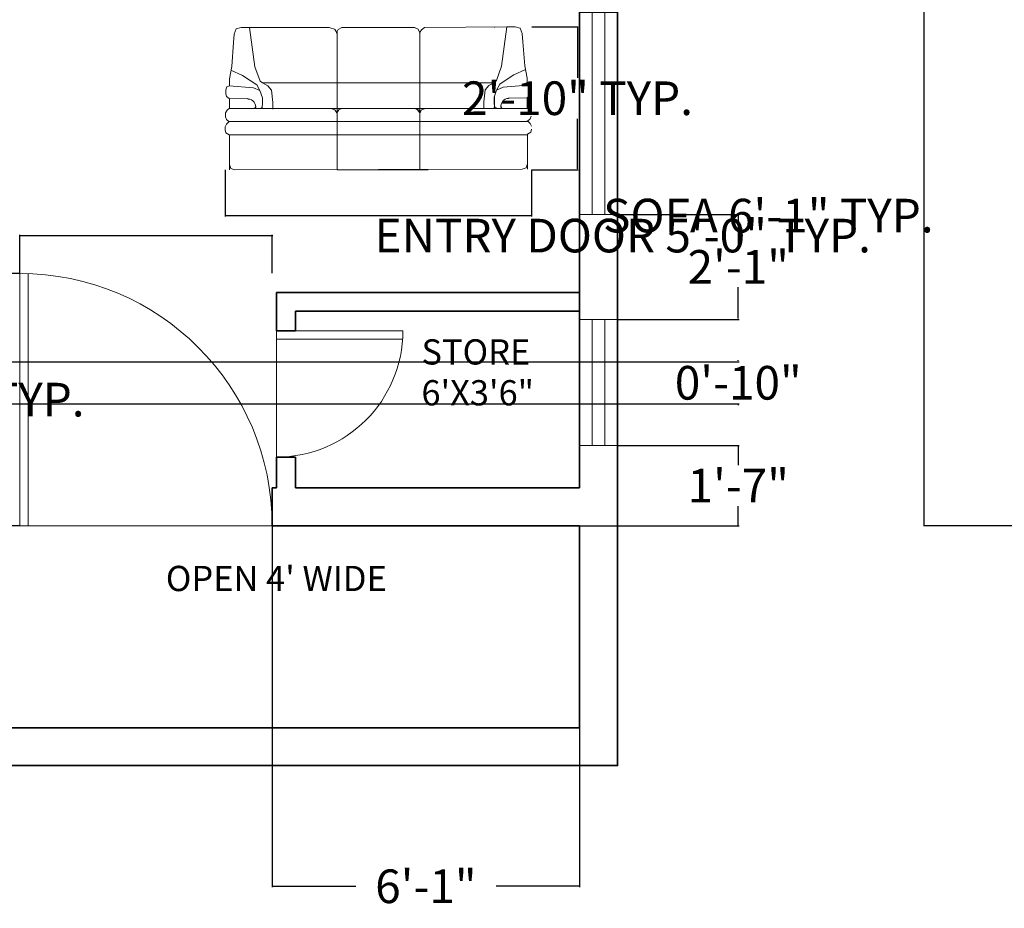
# Model space of a CAD drawing. Units: inches. Extents: x 125 to 976, y 231 to 853.
# Tile 4 of 16: x 324 to 557, y 238 to 449. Entities that reach past the tile are written whole.
import ezdxf

# ---------------------------------------------------------------- set-up
doc = ezdxf.new("R2010")
doc.units = ezdxf.units.IN
doc.header["$MEASUREMENT"] = 0
for name, color, linetype, lineweight in [('A-ANNO-DIMS', 2, 'Continuous', 18), ('A-AREA-IDEN', 7, 'Continuous', 18), ('A-DOOR', 3, 'Continuous', 18), ('A-GLAZ', 4, 'Continuous', 18), ('A-WALL', 7, 'Continuous', 35), ('Furniture', 8, 'Continuous', 15)]:
    doc.layers.add(name, color=color, linetype=linetype, lineweight=lineweight)
doc.styles.get("Standard").update_dxf_attribs({"font": 'italic8.shx'})
doc.dimstyles.get("Standard").update_dxf_attribs({"dimtxt": 8, "dimasz": 0.18, "dimexe": 0.18, "dimexo": 0.0625, "dimgap": 0.09, "dimtad": 0, "dimtih": 1, "dimtoh": 1, "dimdec": 4, "dimzin": 0, "dimdsep": 46, "dimlunit": 3, "dimtxsty": 'Standard', "dimcen": 0.09, "dimclrt": 4, "dimadec": 0, "dimazin": 0, "dimtfac": 1, "dimtdec": 4, "dimtofl": 0, "dimtmove": 0, "dimatfit": 3, "dimfxl": 1, "dimtolj": 1, "dimtzin": 0, "dimarcsym": 0})

# ---------------------------------------------------------------- blocks, each defined once
blk = doc.blocks.new('SOFA-3SEAT')
for p, q in [((2.15, 32.26, -13.5), (2.61, 33.47, -13.5)), ((2.61, 33.47, -13.5), (3.76, 33.83, -13.5)), ((3.76, 33.83, -13.5), (5.77, 33.83, -13.5)), ((5.77, 33.83, -13.5), (24.71, 33.77, -13.5)), ((5.77, 33.83, -13.5), (7.07, 24.49, -13.5)), ((24.71, 33.77, -13.5), (26.18, 33.35, -13.5)), ((26.04, 33.37, -13.5), (26.5, 32.59, -13.5)), ((26.43, 32.53, -13.5), (26.87, 33.35, -13.5)), ((26.58, 32.81, -13.5), (26.58, 0, -13.5)), ((26.87, 33.35, -13.5), (27.73, 33.77, -13.5)), ((27.73, 33.77, -13.5), (44.96, 33.81, -13.5)), ((45.83, 33.4, -13.5), (44.96, 33.81, -13.5)), ((46.26, 32.57, -13.5), (45.83, 33.4, -13.5)), ((46.26, 32.63, -13.5), (46.69, 33.25, -13.5)), ((46.69, 33.25, -13.5), (47.38, 33.77, -13.5)), ((47.38, 33.77, -13.5), (66.92, 33.97, -13.5)), ((63.98, 33.86, -13.5), (63.98, 33.83, -13.5)), ((66.92, 33.97, -13.5), (65.66, 24.62, -13.5)), ((68.93, 33.98, -13.5), (66.92, 33.97, -13.5)), ((70.09, 33.62, -13.5), (68.93, 33.98, -13.5)), ((70.54, 32.42, -13.5), (70.09, 33.62, -13.5)), ((2, 30.21, -13.5), (2.15, 32.26, -13.5)), ((26.46, 32.58, -13.5), (26.52, 32.42, -13.5)), ((46.23, 32.63, -13.5), (46.18, 32.47, -13.5)), ((46.27, 0, -13.5), (46.27, 32.64, -13.5)), ((70.7, 30.37, -13.5), (70.54, 32.42, -13.5)), ((1.55, 24.55, -13.5), (2, 30.21, -13.5)), ((71.18, 24.71, -13.5), (70.7, 30.37, -13.5)), ((0.99, 21.59, -13.5), (1.55, 24.55, -13.5)), ((1.35, 23.64, -13.5), (4.11, 22.38, -13.5)), ((7.07, 24.49, -13.5), (8.28, 21.05, -13.5)), ((65.66, 24.62, -13.5), (64.47, 21.18, -13.5)), ((71.39, 23.81, -13.5), (68.63, 22.53, -13.5)), ((71.76, 21.75, -13.5), (71.18, 24.71, -13.5)), ((0.99, 21.59, -13.5), (0.99, 19.94, -13.5)), ((4.11, 22.38, -13.5), (5.97, 21.23, -13.5)), ((5.97, 21.23, -13.5), (7.53, 20.21, -13.5)), ((64.47, 21.18, -13.5), (63.92, 20.76, -13.5)), ((66.78, 21.37, -13.5), (65.23, 20.34, -13.5)), ((68.63, 22.53, -13.5), (66.78, 21.37, -13.5)), ((71.76, 21.75, -13.5), (71.76, 20.1, -13.5)), ((0.14, 18.15, -13.5), (0.18, 18.99, -13.5)), ((0.18, 18.99, -13.5), (0.38, 19.7, -13.5)), ((0.38, 19.7, -13.5), (0.98, 19.91, -13.5)), ((0.65, 19.79, -13.5), (0.65, 19.8, -13.5)), ((0.96, 19.94, -13.5), (6.7, 19.5, -13.5)), ((6.7, 19.5, -13.5), (8.26, 18.79, -13.5)), ((7.53, 20.21, -13.5), (8.33, 18.64, -13.5)), ((8.26, 18.79, -13.5), (8.83, 17.11, -13.5)), ((8.28, 21.05, -13.5), (8.83, 20.63, -13.5)), ((8.83, 20.63, -13.5), (63.95, 20.63, -13.5)), ((8.83, 20.63, -13.5), (10.14, 19.91, -13.5)), ((8.86, 20.63, -13.5), (8.86, 20.61, -13.5)), ((10.14, 19.91, -13.5), (10.98, 18.9, -13.5)), ((10.98, 18.9, -13.5), (11.34, 16.01, -13.5)), ((61.78, 19.02, -13.5), (61.43, 16.13, -13.5)), ((62.62, 20.03, -13.5), (61.78, 19.02, -13.5)), ((63.92, 20.76, -13.5), (62.62, 20.03, -13.5)), ((63.89, 20.76, -13.5), (63.89, 20.74, -13.5)), ((64.5, 18.92, -13.5), (63.94, 17.24, -13.5)), ((65.23, 20.34, -13.5), (64.43, 18.77, -13.5)), ((66.05, 19.64, -13.5), (64.5, 18.92, -13.5)), ((71.8, 20.1, -13.5), (66.05, 19.64, -13.5)), ((72.37, 19.87, -13.5), (71.78, 20.07, -13.5)), ((72.11, 19.95, -13.5), (72.11, 19.96, -13.5)), ((72.58, 19.16, -13.5), (72.37, 19.87, -13.5)), ((72.62, 18.32, -13.5), (72.58, 19.16, -13.5)), ((0.35, 17.44, -13.5), (0.14, 18.15, -13.5)), ((0.98, 16.94, -13.5), (0.35, 17.44, -13.5)), ((0.98, 16.95, -13.5), (5.28, 16.85, -13.5)), ((0.99, 16.95, -13.5), (0.99, 14.57, -13.5)), ((0.99, 14.57, -13.5), (0.99, 16.93, -13.5)), ((5.51, 16.75, -13.5), (5.27, 16.91, -13.5)), ((8.83, 17.11, -13.5), (8.86, 15.72, -13.5)), ((63.94, 17.24, -13.5), (63.91, 15.85, -13.5)), ((63.98, 17.37, -13.5), (63.98, 14.57, -13.5)), ((67.26, 16.9, -13.5), (67.49, 17.06, -13.5)), ((71.79, 17.11, -13.5), (67.48, 17, -13.5)), ((71.78, 17.11, -13.5), (71.79, 14.73, -13.5)), ((71.79, 14.73, -13.5), (71.78, 17.09, -13.5)), ((71.79, 17.1, -13.5), (72.41, 17.61, -13.5)), ((71.86, 17.15, -13.5), (71.86, 14.57, -13.5)), ((72.41, 17.61, -13.5), (72.62, 18.32, -13.5)), ((0.04, 13.5, -13.5), (0.49, 14.17, -13.5)), ((0.49, 14.17, -13.5), (1.01, 14.59, -13.5)), ((0.99, 14.57, -13.5), (71.86, 14.57, -13.5)), ((0.99, 14.57, -13.5), (0.99, 14.57, -13.5)), ((7.07, 14.84, -13.5), (7.3, 14.56, -13.5)), ((8.66, 14.72, -13.5), (8.26, 14.56, -13.5)), ((8.83, 14.88, -13.5), (8.66, 14.72, -13.5)), ((8.86, 15.75, -13.5), (8.81, 14.86, -13.5)), ((8.89, 14.57, -13.5), (8.89, 14.52, -13.5)), ((11.34, 16.01, -13.5), (11.34, 14.42, -13.5)), ((25.14, 14.53, -13.5), (26.09, 14.22, -13.5)), ((26.09, 14.22, -13.5), (26.52, 13.5, -13.5)), ((26.52, 13.5, -13.5), (27.04, 14.22, -13.5)), ((27.04, 14.22, -13.5), (27.73, 14.53, -13.5)), ((45.74, 14.26, -13.5), (45.05, 14.57, -13.5)), ((45.14, 14.53, -13.5), (46.17, 14.12, -13.5)), ((46.26, 13.54, -13.5), (45.74, 14.26, -13.5)), ((46.17, 14.12, -13.5), (46.26, 13.39, -13.5)), ((46.69, 14.27, -13.5), (46.26, 13.54, -13.5)), ((46.26, 13.39, -13.5), (46.6, 14.12, -13.5)), ((46.6, 14.12, -13.5), (47.29, 14.53, -13.5)), ((47.64, 14.58, -13.5), (46.69, 14.27, -13.5)), ((61.43, 16.13, -13.5), (61.44, 14.54, -13.5)), ((63.88, 14.69, -13.5), (63.88, 14.65, -13.5)), ((63.91, 15.87, -13.5), (63.97, 14.99, -13.5)), ((63.95, 15.01, -13.5), (64.12, 14.85, -13.5)), ((64.12, 14.85, -13.5), (64.51, 14.69, -13.5)), ((65.71, 14.98, -13.5), (65.48, 14.7, -13.5)), ((72.29, 14.34, -13.5), (71.76, 14.75, -13.5)), ((71.79, 14.73, -13.5), (71.79, 14.74, -13.5)), ((72.75, 13.67, -13.5), (72.29, 14.34, -13.5)), ((0.04, 12.58, -13.5), (0.04, 13.5, -13.5)), ((0.31, 11.91, -13.5), (0.04, 12.58, -13.5)), ((0.98, 11.41, -13.5), (0.31, 11.91, -13.5)), ((71.81, 11.57, -13.5), (72.48, 12.08, -13.5)), ((72.48, 12.08, -13.5), (72.75, 12.75, -13.5)), ((0.31, 10.84, -13.5), (0, 10.18, -13.5)), ((0, 10.18, -13.5), (0, 9.47, -13.5)), ((0, 9.47, -13.5), (0.19, 8.77, -13.5)), ((0.98, 11.45, -13.5), (0.31, 10.84, -13.5)), ((71.86, 11.42, -13.5), (0.99, 11.42, -13.5)), ((71.8, 11.42, -13.5), (71.8, 11.58, -13.5)), ((71.82, 11.61, -13.5), (72.49, 11, -13.5)), ((71.86, 11.6, -13.5), (71.86, 11.42, -13.5)), ((71.86, 11.6, -13.5), (71.86, 11.42, -13.5)), ((72.49, 11, -13.5), (72.8, 10.35, -13.5)), ((72.81, 9.64, -13.5), (72.61, 8.93, -13.5)), ((0.19, 8.77, -13.5), (0.98, 8.25, -13.5)), ((0.99, 8.27, -13.5), (71.86, 8.27, -13.5)), ((0.99, 0, -13.5), (0.99, 8.27, -13.5)), ((0.99, 8.27, -13.5), (0.99, 1.21, -13.5)), ((0.99, 8.27, -13.5), (0.99, 0, -13.5)), ((71.82, 8.43, -13.5), (71.81, 8.27, -13.5)), ((71.86, 0.16, -13.5), (71.82, 8.43, -13.5)), ((71.82, 8.43, -13.5), (71.85, 1.37, -13.5)), ((71.86, 0.16, -13.5), (71.82, 8.27, -13.5)), ((72.61, 8.93, -13.5), (71.83, 8.41, -13.5)), ((71.86, 8.43, -13.5), (71.86, 8.27, -13.5)), ((0.99, 1.21, -13.5), (1.35, 0.26, -13.5)), ((1.35, 0.26, -13.5), (2.3, 0, -13.5)), ((2.3, 0, -13.5), (70.55, 0.16, -13.5)), ((71.49, 0.42, -13.5), (70.55, 0.16, -13.5)), ((71.85, 1.37, -13.5), (71.49, 0.42, -13.5)), ((26.58, 0, -13.5), (46.27, 0, -13.5)), ((28.55, 0, -13.5), (48.23, 0, -13.5))]:
    blk.add_line(p, q)
for centre, start, end in [((5.4, 14.95, -13.5), 347.9294, 88.2763), ((67.38, 15.1, -13.5), 91.9867, 192.3335)]:
    blk.add_arc(centre, 1.85, start, end)
blk = doc.blocks.new('WINDOW-48IN')
for p, q in [((0, 0), (0, 48)), ((0, 48), (9, 48)), ((3, 0), (3, 48)), ((6, 0), (6, 48)), ((9, 48), (9, 0)), ((9, 0), (0, 0))]:
    blk.add_line(p, q)
blk = doc.blocks.new('WINDOW-30IN')
for p, q in [((0, 0), (0, 9)), ((0, 9), (30, 9)), ((30, 9), (30, 0)), ((30, 6), (0, 6)), ((30, 3), (0, 3)), ((30, 0), (0, 0))]:
    blk.add_line(p, q)
blk = doc.blocks.new('DOOR-30IN')
for p, q in [((-2, 29.93), (-2, 0)), ((0, 30), (0, 0)), ((0, 0), (-30, 0))]:
    blk.add_line(p, q)
blk.add_arc((0, 0), 30, 90, 180)
blk = doc.blocks.new('DOOR-60IN')
for p, q in [((0, 0), (0, 60)), ((2, 0), (2, 59.97)), ((60, 0), (0, 0))]:
    blk.add_line(p, q)
blk.add_arc((0, 0), 60, 0, 90)
blk = doc.blocks.new('*D42')
at = {"layer": 'A-ANNO-DIMS', "color": 0, "lineweight": -2, "transparency": 16777216}
for p, q in [((372.34, 413.71), (372.34, 402.67)), ((445.15, 413.71), (445.15, 402.67)), ((372.52, 402.85), (444.97, 402.85)), ((445.15, 402.85), (445.33, 402.85))]:
    blk.add_line(p, q, dxfattribs=at)
at = {"layer": 'A-ANNO-DIMS', "color": 0, "transparency": 16777216}
for points in [[(372.52, 402.88), (372.52, 402.82), (372.34, 402.85)], [(444.97, 402.88), (444.97, 402.82), (445.15, 402.85)]]:
    blk.add_solid(points, dxfattribs=at)
at = {"layer": 'Defpoints', "color": 0, "transparency": 16777216}
for p in [(372.34, 413.77), (445.15, 413.77), (445.15, 402.85)]:
    blk.add_point(p, dxfattribs=at)
at = {"layer": 'A-ANNO-DIMS', "color": 4, "transparency": 16777216, "insert": (501.42, 402.85), "char_height": 8, "attachment_point": 5}
blk.add_mtext('\\A1;SOFA 6\'-1" TYP.', dxfattribs=at)
blk = doc.blocks.new('*D43')
at = {"layer": 'A-ANNO-DIMS', "color": 0, "lineweight": -2, "transparency": 16777216}
for p, q in [((445.21, 447.74), (456.25, 447.74)), ((456.07, 447.56), (456.07, 435.61)), ((456.07, 413.95), (456.07, 425.9)), ((445.21, 413.77), (456.25, 413.77))]:
    blk.add_line(p, q, dxfattribs=at)
at = {"layer": 'A-ANNO-DIMS', "color": 0, "transparency": 16777216}
for points in [[(456.04, 447.56), (456.1, 447.56), (456.07, 447.74)], [(456.04, 413.95), (456.1, 413.95), (456.07, 413.77)]]:
    blk.add_solid(points, dxfattribs=at)
at = {"layer": 'Defpoints', "color": 0, "transparency": 16777216}
for p in [(445.15, 447.74), (456.07, 447.74), (445.15, 413.77)]:
    blk.add_point(p, dxfattribs=at)
at = {"layer": 'A-ANNO-DIMS', "color": 4, "transparency": 16777216, "insert": (456.07, 430.76), "char_height": 8, "attachment_point": 5}
blk.add_mtext('\\A1;2\'-10" TYP.', dxfattribs=at)
blk = doc.blocks.new('*D54')
at = {"layer": 'A-ANNO-DIMS', "color": 0, "lineweight": -2, "transparency": 16777216}
for p, q in [((323.51, 389.17), (323.51, 398.28)), ((323.69, 398.1), (383.33, 398.1)), ((383.51, 389.17), (383.51, 398.28)), ((383.51, 398.1), (383.69, 398.1))]:
    blk.add_line(p, q, dxfattribs=at)
at = {"layer": 'A-ANNO-DIMS', "color": 0, "transparency": 16777216}
for points in [[(323.69, 398.13), (323.69, 398.07), (323.51, 398.1)], [(383.33, 398.13), (383.33, 398.07), (383.51, 398.1)]]:
    blk.add_solid(points, dxfattribs=at)
at = {"layer": 'Defpoints', "color": 0, "transparency": 16777216}
for p in [(383.51, 398.1), (323.51, 389.1), (383.51, 389.1)]:
    blk.add_point(p, dxfattribs=at)
at = {"layer": 'A-ANNO-DIMS', "color": 4, "transparency": 16777216, "insert": (466.83, 398.1), "char_height": 8, "attachment_point": 5}
blk.add_mtext('\\A1;ENTRY DOOR 5\'-0" TYP.', dxfattribs=at)
blk = doc.blocks.new('*D55')
at = {"layer": 'A-ANNO-DIMS', "color": 0, "lineweight": -2, "transparency": 16777216}
for p, q in [((323.45, 389.1), (314.33, 389.1)), ((314.51, 388.92), (314.51, 363.96)), ((314.51, 329.28), (314.51, 354.25)), ((323.45, 329.1), (314.33, 329.1))]:
    blk.add_line(p, q, dxfattribs=at)
at = {"layer": 'A-ANNO-DIMS', "color": 0, "transparency": 16777216}
for points in [[(314.48, 388.92), (314.54, 388.92), (314.51, 389.1)], [(314.48, 329.28), (314.54, 329.28), (314.51, 329.1)]]:
    blk.add_solid(points, dxfattribs=at)
at = {"layer": 'Defpoints', "color": 0, "transparency": 16777216}
for p in [(314.51, 389.1), (323.51, 389.1), (323.51, 329.1)]:
    blk.add_point(p, dxfattribs=at)
at = {"layer": 'A-ANNO-DIMS', "color": 4, "transparency": 16777216, "insert": (314.51, 359.1), "char_height": 8, "attachment_point": 5}
blk.add_mtext('\\A1;5\'-0" TYP.', dxfattribs=at)
blk = doc.blocks.new('*D57')
at = {"layer": 'A-ANNO-DIMS', "color": 0, "lineweight": -2, "transparency": 16777216}
for p, q in [((567.13, 812.1), (538.31, 812.1)), ((538.49, 811.92), (538.49, 575.46)), ((538.49, 329.28), (538.49, 565.75)), ((576.13, 329.1), (538.31, 329.1))]:
    blk.add_line(p, q, dxfattribs=at)
at = {"layer": 'A-ANNO-DIMS', "color": 0, "transparency": 16777216}
for points in [[(538.46, 811.92), (538.52, 811.92), (538.49, 812.1)], [(538.46, 329.28), (538.52, 329.28), (538.49, 329.1)]]:
    blk.add_solid(points, dxfattribs=at)
at = {"layer": 'Defpoints', "color": 0, "transparency": 16777216}
for p in [(538.49, 812.1), (567.19, 812.1), (576.19, 329.1)]:
    blk.add_point(p, dxfattribs=at)
at = {"layer": 'A-ANNO-DIMS', "color": 4, "transparency": 16777216, "insert": (538.49, 570.6), "char_height": 8, "attachment_point": 5}
blk.add_mtext('\\A1;40\'-3"', dxfattribs=at)
blk = doc.blocks.new('*D59')
at = {"layer": 'A-ANNO-DIMS', "color": 0, "lineweight": -2, "transparency": 16777216}
for p, q in [((222.641698, 368.104746), (494.459198, 368.104746)), ((494.279198, 368.284746), (494.279198, 368.464746)), ((222.641698, 358.104746), (494.459198, 358.104746)), ((494.279198, 357.924746), (494.279198, 357.744746))]:
    blk.add_line(p, q, dxfattribs=at)
at = {"layer": 'A-ANNO-DIMS', "color": 0, "transparency": 16777216}
for points in [[(494.249198, 368.284746), (494.309198, 368.284746), (494.279198, 368.104746)], [(494.249198, 357.924746), (494.309198, 357.924746), (494.279198, 358.104746)]]:
    blk.add_solid(points, dxfattribs=at)
at = {"layer": 'Defpoints', "color": 0, "transparency": 16777216}
for p in [(222.579198, 368.104746), (494.279198, 368.104746), (222.579198, 358.104746)]:
    blk.add_point(p, dxfattribs=at)
at = {"layer": 'A-ANNO-DIMS', "color": 4, "transparency": 16777216, "insert": (494.279198, 363.104746), "char_height": 8, "attachment_point": 5}
blk.add_mtext('\\A1;0\'-10"', dxfattribs=at)
blk = doc.blocks.new('*D60')
at = {"layer": 'A-ANNO-DIMS', "color": 0, "lineweight": -2, "transparency": 16777216}
for p, q in [((383.51, 329.04), (383.51, 243.22)), ((456.58, 329.04), (456.58, 243.22)), ((383.69, 243.4), (403.39, 243.4)), ((456.4, 243.4), (436.71, 243.4))]:
    blk.add_line(p, q, dxfattribs=at)
at = {"layer": 'A-ANNO-DIMS', "color": 0, "transparency": 16777216}
for points in [[(383.69, 243.43), (383.69, 243.37), (383.51, 243.4)], [(456.4, 243.43), (456.4, 243.37), (456.58, 243.4)]]:
    blk.add_solid(points, dxfattribs=at)
at = {"layer": 'Defpoints', "color": 0, "transparency": 16777216}
for p in [(383.51, 329.1), (456.58, 329.1), (456.58, 243.4)]:
    blk.add_point(p, dxfattribs=at)
at = {"layer": 'A-ANNO-DIMS', "color": 4, "transparency": 16777216, "insert": (420.05, 243.4), "char_height": 8, "attachment_point": 5}
blk.add_mtext('\\A1;6\'-1"', dxfattribs=at)
blk = doc.blocks.new('*D62')
at = {"layer": 'A-ANNO-DIMS', "color": 0, "lineweight": -2, "transparency": 16777216}
for p, q in [((465.64, 348.19), (494.46, 348.19)), ((494.28, 348.01), (494.28, 343.5)), ((494.28, 329.28), (494.28, 333.79)), ((456.64, 329.1), (494.46, 329.1))]:
    blk.add_line(p, q, dxfattribs=at)
at = {"layer": 'A-ANNO-DIMS', "color": 0, "transparency": 16777216}
for points in [[(494.25, 348.01), (494.31, 348.01), (494.28, 348.19)], [(494.25, 329.28), (494.31, 329.28), (494.28, 329.1)]]:
    blk.add_solid(points, dxfattribs=at)
at = {"layer": 'Defpoints', "color": 0, "transparency": 16777216}
for p in [(465.58, 348.19), (494.28, 348.19), (456.58, 329.1)]:
    blk.add_point(p, dxfattribs=at)
at = {"layer": 'A-ANNO-DIMS', "color": 4, "transparency": 16777216, "insert": (494.28, 338.65), "char_height": 8, "attachment_point": 5}
blk.add_mtext('\\A1;1\'-7"', dxfattribs=at)
blk = doc.blocks.new('*D63')
at = {"layer": 'A-ANNO-DIMS', "color": 0, "lineweight": -2, "transparency": 16777216}
for p, q in [((465.64, 403.13), (494.46, 403.13)), ((494.28, 402.95), (494.28, 395.51)), ((494.28, 378.37), (494.28, 385.8)), ((465.64, 378.19), (494.46, 378.19))]:
    blk.add_line(p, q, dxfattribs=at)
at = {"layer": 'A-ANNO-DIMS', "color": 0, "transparency": 16777216}
for points in [[(494.25, 402.95), (494.31, 402.95), (494.28, 403.13)], [(494.25, 378.37), (494.31, 378.37), (494.28, 378.19)]]:
    blk.add_solid(points, dxfattribs=at)
at = {"layer": 'Defpoints', "color": 0, "transparency": 16777216}
for p in [(465.58, 403.13), (494.28, 403.13), (465.58, 378.19)]:
    blk.add_point(p, dxfattribs=at)
at = {"layer": 'A-ANNO-DIMS', "color": 4, "transparency": 16777216, "insert": (494.28, 390.66), "char_height": 8, "attachment_point": 5}
blk.add_mtext('\\A1;2\'-1"', dxfattribs=at)

msp = doc.modelspace()

# ---------------------------------------------------------------- linework, layer by layer
at = {"layer": 'A-WALL'}
for p, q in [((456.5792, 338.10475), (456.5792, 494.10475)), ((384.5792, 384.60475), (456.5792, 384.60475)), ((384.5792, 375.45103), (384.5792, 384.60475)), ((389.0792, 380.10475), (456.5792, 380.10475)), ((389.0792, 375.45103), (389.0792, 380.10475)), ((389.0792, 375.45103), (384.5792, 375.45103)), ((384.5792, 338.10475), (384.5792, 345.45103)), ((389.0792, 345.45103), (384.5792, 345.45103)), ((389.0792, 338.10475), (389.0792, 345.45103)), ((383.51392, 338.10475), (383.51392, 329.10475)), ((383.51392, 338.10475), (384.5792, 338.10475)), ((389.0792, 338.10475), (456.5792, 338.10475)), ((383.51392, 329.10475), (456.5792, 329.10475)), ((456.5792, 281.10475), (456.5792, 329.10475)), ((186.5792, 281.10475), (456.5792, 281.10475))]:
    msp.add_line(p, q, dxfattribs=at)
msp.add_lwpolyline([(177.5792, 272.10475), (465.5792, 272.10475), (465.5792, 812.10475), (177.5792, 812.10475)], close=True, dxfattribs=at)

# ---------------------------------------------------------------- block references
at = {"layer": 'A-DOOR'}
msp.add_blockref('DOOR-60IN', (323.51392, 329.10475), dxfattribs=at)
at = {"layer": 'A-DOOR', "extrusion": (0, 0, -1), "zscale": -1, "rotation": 89.99999999999989}
msp.add_blockref('DOOR-30IN', (-384.5792, 375.45103), dxfattribs=at)
at = {"layer": 'A-GLAZ'}
msp.add_blockref('WINDOW-48IN', (456.57633, 403.12016), dxfattribs=at)
at = {"layer": 'A-GLAZ', "rotation": 270.0000000000005}
msp.add_blockref('WINDOW-30IN', (456.57445, 378.18295), dxfattribs=at)
at = {"layer": 'Furniture'}
msp.add_blockref('SOFA-3SEAT', (372.34653, 413.76815), dxfattribs=at)

# ---------------------------------------------------------------- texts
at = {"layer": 'A-AREA-IDEN'}
for s, p in [('STORE', (418.98531, 367.44524)), ('6\'X3\'6"', (418.98531, 357.73095)), ("OPEN 4' WIDE", (358.24139, 313.57942))]:
    msp.add_text(s, height=6, dxfattribs=at).set_placement(p)

# ---------------------------------------------------------------- dimensions: what is measured, and where the dimension line sits
at = {"layer": 'A-ANNO-DIMS'}
for base, p1, p2, picture, middle in [((538.49287, 812.10475), (576.19287, 329.10475), (567.19287, 812.10475), '*D57', (538.49287, 570.60475)), ((494.2792, 403.12515), (465.5792, 378.18698), (465.5792, 403.12515), '*D63', (494.2792, 390.65607)), ((494.2792, 368.10475), (222.5792, 358.10475), (222.5792, 368.10475), '*D59', (494.2792, 363.10475)), ((494.2792, 348.18698), (456.5792, 329.10475), (465.5792, 348.18698), '*D62', (494.2792, 338.64586))]:
    dim = msp.add_linear_dim(base=base, p1=p1, p2=p2, angle=90, dimstyle='Standard', override={"dimdec": 1, "dimlfac": 1, "dimrnd": 0, "dimzin": 1, "dimdsep": 46, "dimlunit": 4, "dimfrac": 2}, dxfattribs=at)
    dim.commit()
    dim.dimension.update_dxf_attribs({"geometry": picture, "text_midpoint": middle})
for base, p1, p2, picture, middle in [((456.07365, 447.74434), (445.15216, 413.76764), (445.15216, 447.74434), '*D43', (456.07365, 430.75599)), ((314.51392, 389.10475), (323.51392, 329.10475), (323.51392, 389.10475), '*D55', (314.51392, 359.10475))]:
    dim = msp.add_linear_dim(base=base, p1=p1, p2=p2, angle=90, text='<> TYP.', dimstyle='Standard', override={"dimdec": 1, "dimlfac": 1, "dimrnd": 0, "dimzin": 1, "dimdsep": 46, "dimlunit": 4, "dimfrac": 2}, dxfattribs=at)
    dim.commit()
    dim.dimension.update_dxf_attribs({"geometry": picture, "text_midpoint": middle})
for base, p1, p2, text, picture, middle in [((383.51392, 398.10475), (323.51392, 389.10475), (383.51392, 389.10475), 'ENTRY DOOR <> TYP.', '*D54', (466.83154, 398.10475)), ((445.15216, 402.84615), (372.34223, 413.76764), (445.15216, 413.76764), 'SOFA <> TYP.', '*D42', (501.42216, 402.84615))]:
    dim = msp.add_linear_dim(base=base, p1=p1, p2=p2, text=text, dimstyle='Standard', override={"dimdec": 1, "dimlfac": 1, "dimrnd": 0, "dimzin": 1, "dimdsep": 46, "dimlunit": 4, "dimfrac": 2}, dxfattribs=at)
    dim.commit()
    dim.dimension.update_dxf_attribs({"geometry": picture, "text_midpoint": middle})
dim = msp.add_linear_dim(base=(456.5792, 243.40475), p1=(383.51392, 329.10475), p2=(456.5792, 329.10475), dimstyle='Standard', override={"dimdec": 1, "dimlfac": 1, "dimrnd": 0, "dimzin": 1, "dimdsep": 46, "dimlunit": 4, "dimfrac": 2}, dxfattribs=at)
dim.commit()
dim.dimension.update_dxf_attribs({"geometry": '*D60', "text_midpoint": (420.04656, 243.40475)})

doc.saveas('drawing.dxf')
